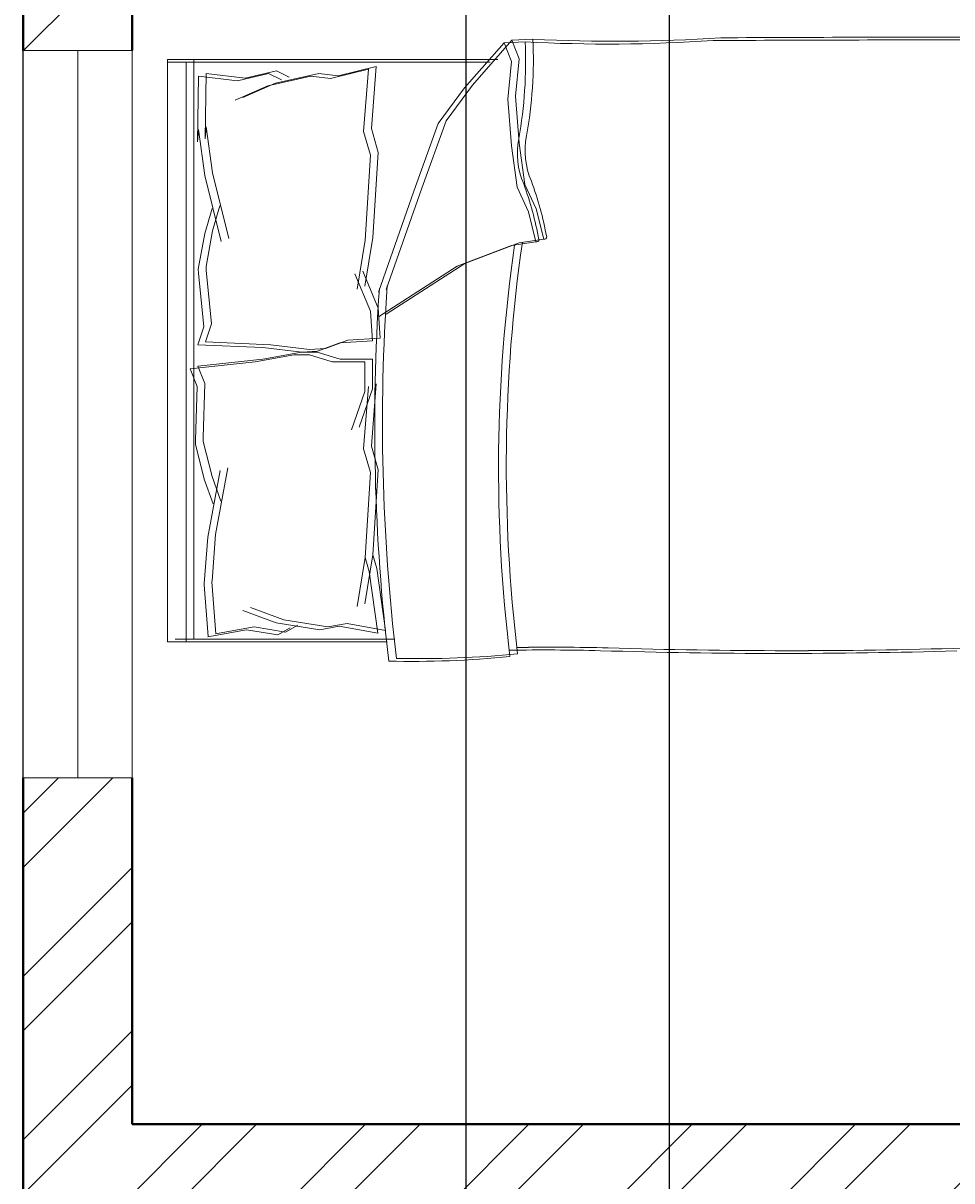
# Model space of a CAD drawing. Units: inches. Extents: x 1601 to 2297, y 1496 to 2631.
# Tile 33 of 57: x 1686 to 1763, y 2141 to 2236. Entities that reach past the tile are written whole.
import ezdxf

# ---------------------------------------------------------------- set-up
doc = ezdxf.new("R2010")
doc.units = ezdxf.units.IN
for name, color, linetype, lineweight in [('A-ANNO-DIMS', 2, 'Continuous', 18), ('A-FURN', 8, 'Continuous', 18), ('A-GLAZ', 161, 'Continuous', 20), ('A-WALL', 7, 'Continuous', 40), ('A-WALL-PATT', 215, 'Continuous', 13)]:
    doc.layers.add(name, color=color, linetype=linetype, lineweight=lineweight)
doc.styles.get("Standard").update_dxf_attribs({"font": 'arial.ttf'})
doc.dimstyles.get("Standard").update_dxf_attribs({"dimtxt": 0.18, "dimasz": 0.18, "dimexe": 0.18, "dimexo": 0.0625, "dimgap": 0.09, "dimtad": 0, "dimtih": 1, "dimtoh": 1, "dimdec": 4, "dimzin": 0, "dimdsep": 46, "dimtxsty": 'Standard', "dimcen": 0.09, "dimadec": 0, "dimazin": 0, "dimtfac": 1, "dimtdec": 4, "dimtofl": 0, "dimtmove": 0, "dimatfit": 3, "dimfxl": 1, "dimtolj": 1, "dimtzin": 0, "dimarcsym": 0})

# ---------------------------------------------------------------- blocks, each defined once
blk = doc.blocks.new('BED-DOUBLE')
for p, q in [((27.746, 52.867), (24.495, 49.162)), ((27.746, 52.867), (24.495, 49.162)), ((27.746, 52.867), (24.495, 49.162)), ((27.746, 52.867), (24.495, 49.162)), ((28.385, 53.096), (25.135, 49.39)), ((28.385, 53.096), (25.135, 49.39)), ((28.385, 53.096), (25.135, 49.39)), ((28.385, 53.096), (25.135, 49.39)), ((29.49, 52.947), (27.746, 52.867, 3.871)), ((29.49, 52.947), (27.746, 52.867, 3.871)), ((29.49, 52.947), (27.746, 52.867, 3.871)), ((29.49, 52.947), (27.746, 52.867, 3.871)), ((28.365, 51.33), (27.746, 52.867)), ((28.365, 51.33), (27.746, 52.867)), ((28.365, 51.33), (27.746, 52.867)), ((28.365, 51.33), (27.746, 52.867)), ((30.13, 53.175), (28.385, 53.096, 3.871)), ((30.13, 53.175), (28.385, 53.096, 3.871)), ((30.13, 53.175), (28.385, 53.096, 3.871)), ((30.13, 53.175), (28.385, 53.096, 3.871)), ((29.004, 51.559), (28.385, 53.096)), ((29.004, 51.558), (28.385, 53.096)), ((29.004, 51.559), (28.385, 53.096)), ((29.004, 51.558), (28.385, 53.096)), ((28.695, 48.461), (29.004, 51.559)), ((28.695, 48.461), (29.004, 51.559)), ((28.695, 48.461), (29.004, 51.558)), ((28.695, 48.461), (29.004, 51.558)), ((0, 51.494), (0.639, 51.493)), ((0, 3.475), (0, 51.494)), ((0, 51.494), (0.639, 51.493)), ((0, 3.475), (0, 51.494)), ((0, 51.265), (26.61, 51.265)), ((0, 51.265), (26.61, 51.265)), ((0, 51.265), (26.61, 51.265)), ((0, 51.265), (26.61, 51.265)), ((0.639, 51.494), (27.249, 51.494)), ((0.639, 51.494), (27.249, 51.494)), ((0.639, 51.493), (27.249, 51.493)), ((0.639, 51.493), (27.249, 51.493)), ((1.533, 3.475), (1.533, 51.265)), ((1.533, 3.475), (1.533, 51.265)), ((1.533, 3.475), (1.533, 51.265)), ((1.533, 3.475), (1.533, 51.265)), ((2.173, 3.703), (2.173, 51.494)), ((2.173, 3.703), (2.173, 51.494)), ((2.173, 3.703), (2.173, 51.493)), ((2.173, 3.703), (2.173, 51.493)), ((16.573, 50.698), (13.434, 49.923)), ((16.573, 50.698), (13.434, 49.922)), ((16.573, 50.698), (13.434, 49.923)), ((16.573, 50.698), (13.434, 49.922)), ((17.212, 50.926), (14.073, 50.151)), ((17.212, 50.926), (14.073, 50.151)), ((17.212, 50.926), (14.073, 50.151)), ((17.212, 50.926), (14.073, 50.151)), ((16.169, 45.566), (16.573, 50.698)), ((16.169, 45.566), (16.573, 50.698)), ((16.169, 45.566), (16.573, 50.698)), ((16.169, 45.566), (16.573, 50.698)), ((16.808, 45.795), (17.212, 50.926)), ((16.808, 45.794), (17.212, 50.926)), ((16.808, 45.795), (17.212, 50.926)), ((16.808, 45.794), (17.212, 50.926)), ((28.055, 48.233), (28.365, 51.33)), ((28.055, 48.233), (28.365, 51.33)), ((28.055, 48.233), (28.365, 51.33)), ((28.055, 48.233), (28.365, 51.33)), ((2.557, 50.112), (2.46, 44.709)), ((2.557, 50.112), (2.46, 44.709)), ((2.557, 50.111), (2.46, 44.709)), ((2.557, 50.111), (2.46, 44.709)), ((2.557, 50.112), (5.768, 49.733)), ((2.557, 50.112), (5.768, 49.733)), ((2.557, 50.111), (5.768, 49.733)), ((2.557, 50.111), (5.768, 49.733)), ((3.196, 50.34), (3.099, 44.938)), ((3.196, 50.34), (3.099, 44.938)), ((3.196, 50.34), (3.099, 44.938)), ((3.196, 50.34), (3.099, 44.938)), ((3.196, 50.34), (6.407, 49.961)), ((3.196, 50.34), (6.407, 49.961)), ((3.196, 50.34), (6.407, 49.961)), ((3.196, 50.34), (6.407, 49.961)), ((5.768, 49.733), (8.338, 50.328)), ((5.768, 49.733), (8.338, 50.328)), ((5.768, 49.733), (8.338, 50.328)), ((5.768, 49.733), (8.338, 50.328)), ((6.407, 49.961), (8.977, 50.557)), ((6.407, 49.961), (8.977, 50.557)), ((6.407, 49.961), (8.977, 50.556)), ((6.407, 49.961), (8.977, 50.556)), ((11.829, 50.112), (8.257, 49.309)), ((11.829, 50.112), (8.257, 49.309)), ((11.829, 50.112), (8.257, 49.309)), ((11.829, 50.112), (8.257, 49.309)), ((8.338, 50.328), (9.384, 49.814)), ((8.338, 50.328), (9.384, 49.814)), ((8.338, 50.328), (9.384, 49.814)), ((8.338, 50.328), (9.384, 49.814)), ((12.468, 50.34), (8.896, 49.538)), ((12.468, 50.34), (8.896, 49.537)), ((12.468, 50.34), (8.896, 49.538)), ((12.468, 50.34), (8.896, 49.537)), ((8.977, 50.557), (10.024, 50.043)), ((8.977, 50.557), (10.024, 50.043)), ((8.977, 50.556), (10.024, 50.042)), ((8.977, 50.556), (10.024, 50.042)), ((13.434, 49.923), (11.829, 50.112)), ((13.434, 49.922), (11.829, 50.112)), ((13.434, 49.923), (11.829, 50.112)), ((13.434, 49.922), (11.829, 50.112)), ((14.073, 50.151), (12.468, 50.34)), ((14.073, 50.151), (12.468, 50.34)), ((14.073, 50.151), (12.468, 50.34)), ((14.073, 50.151), (12.468, 50.34)), ((8.257, 49.309), (5.578, 48.128)), ((8.257, 49.309), (5.578, 48.128)), ((8.257, 49.309), (5.578, 48.128)), ((8.257, 49.309), (5.578, 48.128)), ((8.896, 49.538), (6.218, 48.356)), ((8.896, 49.538), (6.218, 48.356)), ((8.896, 49.537), (6.218, 48.356)), ((8.896, 49.537), (6.218, 48.356)), ((24.495, 49.162), (22.329, 46.219)), ((24.495, 49.162), (22.329, 46.219)), ((24.495, 49.162), (22.329, 46.219)), ((24.495, 49.162), (22.329, 46.219)), ((25.135, 49.39), (22.968, 46.448)), ((25.135, 49.39), (22.968, 46.448)), ((25.135, 49.39), (22.968, 46.448)), ((25.135, 49.39), (22.968, 46.448)), ((28.365, 44.361), (28.055, 48.233)), ((28.365, 44.361), (28.055, 48.233)), ((28.365, 44.361), (28.055, 48.233)), ((28.365, 44.361), (28.055, 48.233)), ((29.004, 44.589), (28.695, 48.461)), ((29.004, 44.589), (28.695, 48.461)), ((29.004, 44.589), (28.695, 48.461)), ((29.004, 44.589), (28.695, 48.461)), ((3.099, 44.938), (3.181, 45.941)), ((3.099, 44.938), (3.181, 45.941)), ((3.099, 44.938), (3.181, 45.94)), ((3.099, 44.938), (3.181, 45.94)), ((3.181, 45.941), (3.709, 42.143)), ((3.181, 45.941), (3.709, 42.143)), ((3.181, 45.94), (3.709, 42.142)), ((3.181, 45.94), (3.709, 42.142)), ((22.329, 46.219), (20.316, 40.644)), ((22.329, 46.219), (20.316, 40.644)), ((22.329, 46.219), (20.317, 40.644)), ((22.329, 46.219), (20.317, 40.644)), ((22.968, 46.448), (20.956, 40.872)), ((22.968, 46.448), (20.956, 40.872)), ((22.968, 46.448), (20.956, 40.872)), ((22.968, 46.448), (20.956, 40.872)), ((2.46, 44.709), (2.542, 45.712)), ((2.46, 44.709), (2.542, 45.712)), ((2.46, 44.709), (2.542, 45.712)), ((2.46, 44.709), (2.542, 45.712)), ((2.542, 45.712), (3.069, 41.914)), ((2.542, 45.712), (3.069, 41.914)), ((2.542, 45.712), (3.069, 41.914)), ((2.542, 45.712), (3.069, 41.914)), ((16.726, 43.606), (16.169, 45.566)), ((16.726, 43.606), (16.169, 45.566)), ((16.726, 43.606), (16.169, 45.566)), ((16.726, 43.606), (16.169, 45.566)), ((17.365, 43.834), (16.808, 45.795)), ((17.365, 43.834), (16.808, 45.795)), ((17.365, 43.834), (16.808, 45.794)), ((17.365, 43.834), (16.808, 45.794)), ((28.829, 40.954), (28.365, 44.361)), ((28.829, 40.953), (28.365, 44.361)), ((28.829, 40.954), (28.365, 44.361)), ((28.829, 40.953), (28.365, 44.361)), ((29.468, 41.182), (29.004, 44.589)), ((29.469, 41.182), (29.004, 44.589)), ((29.468, 41.182), (29.004, 44.589)), ((29.469, 41.182), (29.004, 44.589)), ((16.295, 36.596), (16.726, 43.606)), ((16.295, 36.596), (16.726, 43.606)), ((16.295, 36.596), (16.726, 43.606)), ((16.295, 36.596), (16.726, 43.606)), ((16.934, 36.824), (17.365, 43.834)), ((16.934, 36.824), (17.365, 43.834)), ((16.934, 36.824), (17.365, 43.834)), ((16.934, 36.824), (17.365, 43.834)), ((3.709, 42.143), (5.061, 36.723)), ((3.709, 42.143), (5.061, 36.723)), ((3.709, 42.142), (5.061, 36.723)), ((3.709, 42.142), (5.061, 36.723)), ((3.069, 41.914), (4.422, 36.495)), ((3.069, 41.914), (4.422, 36.495)), ((3.069, 41.914), (4.422, 36.495)), ((3.069, 41.914), (4.422, 36.495)), ((30.397, 39.169), (29.468, 41.182)), ((30.397, 39.169), (29.468, 41.182)), ((30.397, 39.168), (29.469, 41.182)), ((30.397, 39.168), (29.469, 41.182)), ((20.316, 40.644), (17.383, 32.306)), ((20.317, 40.644), (17.383, 32.306)), ((20.316, 40.644), (17.383, 32.306)), ((20.317, 40.644), (17.383, 32.306)), ((20.956, 40.872), (18.022, 32.534)), ((20.956, 40.872), (18.022, 32.534)), ((20.956, 40.872), (18.022, 32.534)), ((20.956, 40.872), (18.022, 32.534)), ((29.758, 38.94), (28.829, 40.954)), ((29.758, 38.94), (28.829, 40.954)), ((29.758, 38.94), (28.829, 40.953)), ((29.758, 38.94), (28.829, 40.953)), ((3.673, 39.2), (3.078, 37.135)), ((3.673, 39.2), (3.078, 37.135)), ((3.673, 39.2), (3.078, 37.135)), ((3.673, 39.2), (3.078, 37.135)), ((4.313, 39.428), (3.717, 37.363)), ((4.313, 39.428), (3.717, 37.363)), ((4.313, 39.428), (3.718, 37.363)), ((4.313, 39.428), (3.718, 37.363)), ((31.016, 36.691), (30.397, 39.169)), ((31.016, 36.691), (30.397, 39.169)), ((31.016, 36.691), (30.397, 39.168)), ((31.016, 36.691), (30.397, 39.168)), ((30.377, 36.462), (29.758, 38.94)), ((30.377, 36.462), (29.758, 38.94)), ((30.377, 36.462), (29.758, 38.94)), ((30.377, 36.462), (29.758, 38.94)), ((3.717, 37.363), (3.176, 34.433)), ((3.718, 37.363), (3.176, 34.433)), ((3.717, 37.363), (3.176, 34.433)), ((3.718, 37.363), (3.176, 34.433)), ((3.078, 37.135), (2.537, 34.204)), ((3.078, 37.135), (2.537, 34.204)), ((3.078, 37.135), (2.537, 34.204)), ((3.078, 37.135), (2.537, 34.204)), ((15.628, 32.564), (16.295, 36.596)), ((15.628, 32.564), (16.295, 36.596)), ((15.628, 32.564), (16.295, 36.596)), ((15.628, 32.564), (16.295, 36.596)), ((16.268, 32.792), (16.934, 36.824)), ((16.268, 32.792), (16.934, 36.824)), ((16.268, 32.792), (16.934, 36.824)), ((16.268, 32.792), (16.934, 36.824)), ((24.516, 34.677), (29.004, 36.381)), ((24.516, 34.677), (29.004, 36.381)), ((24.516, 34.677), (29.004, 36.381)), ((24.516, 34.677), (29.004, 36.381)), ((28.365, 36.153), (30.377, 36.462)), ((28.365, 36.152), (30.377, 36.462)), ((28.365, 36.153), (30.377, 36.462)), ((28.365, 36.152), (30.377, 36.462)), ((29.004, 36.381), (31.016, 36.691)), ((29.004, 36.381), (31.016, 36.691)), ((29.004, 36.381), (31.016, 36.691)), ((29.004, 36.381), (31.016, 36.691)), ((23.876, 34.449), (28.365, 36.153)), ((23.876, 34.449), (28.365, 36.153)), ((23.876, 34.449), (28.365, 36.152)), ((23.876, 34.449), (28.365, 36.152)), ((3.176, 34.433), (3.196, 34.112)), ((3.176, 34.433), (3.196, 34.112)), ((3.176, 34.433), (3.196, 34.112)), ((3.176, 34.433), (3.196, 34.112)), ((17.383, 30.259), (23.876, 34.449)), ((17.383, 30.259), (23.876, 34.449)), ((17.383, 30.259), (23.876, 34.449)), ((17.383, 30.259), (23.876, 34.449)), ((18.022, 30.487), (24.516, 34.677)), ((18.022, 30.487), (24.516, 34.677)), ((18.022, 30.487), (24.516, 34.677)), ((18.022, 30.487), (24.516, 34.677)), ((2.537, 34.204), (2.557, 33.883)), ((2.537, 34.204), (2.557, 33.883)), ((2.537, 34.204), (2.557, 33.883)), ((2.537, 34.204), (2.557, 33.883)), ((2.557, 33.883), (2.979, 29.456)), ((2.557, 33.883), (2.979, 29.455)), ((2.557, 33.883), (2.979, 29.456)), ((2.557, 33.883), (2.979, 29.455)), ((3.196, 34.112), (3.618, 29.684)), ((3.196, 34.112), (3.618, 29.684)), ((3.196, 34.112), (3.618, 29.684)), ((3.196, 34.112), (3.618, 29.684)), ((16.739, 30.75), (15.454, 33.821)), ((16.739, 30.75), (15.454, 33.821)), ((16.739, 30.75), (15.454, 33.82)), ((16.739, 30.75), (15.454, 33.82)), ((17.379, 30.978), (16.094, 34.049)), ((17.379, 30.978), (16.094, 34.049)), ((17.379, 30.978), (16.094, 34.049)), ((17.379, 30.978), (16.094, 34.049)), ((16.893, 28.297), (16.739, 30.75)), ((16.893, 28.297), (16.739, 30.75)), ((16.893, 28.297), (16.739, 30.75)), ((16.893, 28.297), (16.739, 30.75)), ((17.532, 28.526), (17.379, 30.978)), ((17.532, 28.525), (17.379, 30.978)), ((17.532, 28.526), (17.379, 30.978)), ((17.532, 28.525), (17.379, 30.978)), ((3.618, 29.684), (3.131, 28.205)), ((3.618, 29.684), (3.131, 28.205)), ((3.618, 29.684), (3.131, 28.205)), ((3.618, 29.684), (3.131, 28.205)), ((2.979, 29.456), (2.492, 27.977)), ((2.979, 29.456), (2.492, 27.977)), ((2.979, 29.455), (2.492, 27.976)), ((2.979, 29.455), (2.492, 27.976)), ((2.492, 27.977), (7.867, 27.733)), ((2.492, 27.977), (7.867, 27.733)), ((2.492, 27.976), (7.867, 27.733)), ((2.492, 27.976), (7.867, 27.733)), ((3.131, 28.205), (8.506, 27.962)), ((3.131, 28.205), (8.506, 27.961)), ((3.131, 28.205), (8.506, 27.962)), ((3.131, 28.205), (8.506, 27.961)), ((7.867, 27.733), (11.078, 27.355)), ((7.867, 27.733), (11.078, 27.354)), ((7.867, 27.733), (11.078, 27.355)), ((7.867, 27.733), (11.078, 27.354)), ((8.506, 27.962), (11.717, 27.583)), ((8.506, 27.962), (11.717, 27.583)), ((8.506, 27.961), (11.717, 27.583)), ((8.506, 27.961), (11.717, 27.583)), ((12.377, 27.436), (14.216, 28.13)), ((12.377, 27.436), (14.217, 28.13)), ((12.377, 27.436), (14.216, 28.13)), ((12.377, 27.436), (14.217, 28.13)), ((13.016, 27.664), (14.856, 28.359)), ((13.016, 27.664), (14.856, 28.359)), ((13.016, 27.664), (14.856, 28.358)), ((13.016, 27.664), (14.856, 28.358)), ((14.216, 28.13), (16.893, 28.297)), ((14.216, 28.13), (16.893, 28.297)), ((14.217, 28.13), (16.893, 28.297)), ((14.217, 28.13), (16.893, 28.297)), ((14.856, 28.359), (17.532, 28.526)), ((14.856, 28.359), (17.532, 28.526)), ((14.856, 28.358), (17.532, 28.525)), ((14.856, 28.358), (17.532, 28.525)), ((2.509, 26.211), (7.859, 26.789)), ((2.509, 26.21), (7.859, 26.789)), ((2.509, 26.211), (7.859, 26.789)), ((2.509, 26.21), (7.859, 26.789)), ((7.22, 26.561), (10.401, 27.139)), ((7.22, 26.56), (10.401, 27.139)), ((7.22, 26.561), (10.401, 27.139)), ((7.22, 26.56), (10.401, 27.139)), ((7.859, 26.789), (11.04, 27.367)), ((7.859, 26.789), (11.04, 27.367)), ((7.859, 26.789), (11.04, 27.367)), ((7.859, 26.789), (11.04, 27.367)), ((10.401, 27.139), (11.702, 27.139)), ((10.401, 27.139), (11.702, 27.139)), ((10.401, 27.139), (11.702, 27.139)), ((10.401, 27.139), (11.702, 27.139)), ((11.04, 27.367), (12.341, 27.367)), ((11.04, 27.367), (12.341, 27.367)), ((11.04, 27.367), (12.341, 27.367)), ((11.04, 27.367), (12.341, 27.367)), ((11.078, 27.355), (12.377, 27.436)), ((11.078, 27.354), (12.377, 27.436)), ((11.078, 27.355), (12.377, 27.436)), ((11.078, 27.354), (12.377, 27.436)), ((11.702, 27.139), (13.582, 26.561)), ((11.702, 27.139), (13.582, 26.56)), ((11.702, 27.139), (13.582, 26.561)), ((11.702, 27.139), (13.582, 26.56)), ((11.717, 27.583), (13.016, 27.664)), ((11.717, 27.583), (13.016, 27.664)), ((11.717, 27.583), (13.016, 27.664)), ((11.717, 27.583), (13.016, 27.664)), ((12.341, 27.367), (14.221, 26.789)), ((12.341, 27.367), (14.221, 26.789)), ((12.341, 27.367), (14.221, 26.789)), ((12.341, 27.367), (14.221, 26.789)), ((14.221, 26.789), (16.902, 26.789)), ((14.221, 26.789), (16.902, 26.789)), ((14.221, 26.789), (16.902, 26.789)), ((14.221, 26.789), (16.902, 26.789)), ((16.902, 26.789), (16.902, 24.332)), ((16.902, 26.789), (16.902, 24.331)), ((16.902, 26.789), (16.902, 24.332)), ((16.902, 26.789), (16.902, 24.331)), ((1.87, 25.982), (7.22, 26.561)), ((1.87, 25.982), (7.22, 26.561)), ((1.87, 25.982), (7.22, 26.56)), ((1.87, 25.982), (7.22, 26.56)), ((2.448, 24.537), (1.87, 25.982)), ((2.448, 24.537), (1.87, 25.982)), ((2.448, 24.537), (1.87, 25.982)), ((2.448, 24.537), (1.87, 25.982)), ((3.088, 24.765), (2.509, 26.211)), ((3.088, 24.765), (2.509, 26.211)), ((3.088, 24.765), (2.509, 26.21)), ((3.088, 24.765), (2.509, 26.21)), ((13.582, 26.561), (16.263, 26.561)), ((13.582, 26.561), (16.263, 26.561)), ((13.582, 26.56), (16.263, 26.56)), ((13.582, 26.56), (16.263, 26.56)), ((16.263, 26.561), (16.263, 24.103)), ((16.263, 26.561), (16.263, 24.103)), ((16.263, 26.56), (16.263, 24.103)), ((16.263, 26.56), (16.263, 24.103)), ((2.304, 20.091), (2.448, 24.537)), ((2.304, 20.091), (2.448, 24.537)), ((2.304, 20.091), (2.448, 24.537)), ((2.304, 20.091), (2.448, 24.537)), ((2.943, 20.32), (3.088, 24.765)), ((2.943, 20.319), (3.088, 24.765)), ((2.943, 20.32), (3.088, 24.765)), ((2.943, 20.319), (3.088, 24.765)), ((16.263, 24.103), (15.172, 20.959)), ((16.263, 24.103), (15.172, 20.958)), ((16.263, 24.103), (15.172, 20.959)), ((16.263, 24.103), (15.172, 20.958)), ((16.902, 24.332), (15.811, 21.187)), ((16.902, 24.332), (15.811, 21.187)), ((16.902, 24.331), (15.811, 21.187)), ((16.902, 24.331), (15.811, 21.187)), ((16.169, 19.384), (16.573, 24.516)), ((16.169, 19.384), (16.573, 24.516)), ((16.169, 19.383), (16.573, 24.515)), ((16.169, 19.383), (16.573, 24.515)), ((16.808, 19.612), (17.212, 24.744)), ((16.808, 19.612), (17.212, 24.744)), ((16.808, 19.612), (17.212, 24.744)), ((16.808, 19.612), (17.212, 24.744)), ((2.304, 19.77), (2.304, 20.091)), ((2.304, 19.769), (2.304, 20.091)), ((2.304, 19.77), (2.304, 20.091)), ((2.304, 19.769), (2.304, 20.091)), ((2.943, 19.998), (2.943, 20.32)), ((2.943, 19.998), (2.943, 20.32)), ((2.943, 19.998), (2.943, 20.319)), ((2.943, 19.998), (2.943, 20.319)), ((3.027, 16.878), (2.304, 19.77)), ((3.027, 16.878), (2.304, 19.77)), ((3.027, 16.878), (2.304, 19.769)), ((3.027, 16.878), (2.304, 19.769)), ((3.666, 17.107), (2.943, 19.998)), ((3.666, 17.107), (2.943, 19.998)), ((3.666, 17.107), (2.943, 19.998)), ((3.666, 17.107), (2.943, 19.998)), ((16.726, 17.423), (16.169, 19.384)), ((16.726, 17.423), (16.169, 19.384)), ((16.726, 17.423), (16.169, 19.383)), ((16.726, 17.423), (16.169, 19.383)), ((17.365, 17.652), (16.808, 19.612)), ((17.365, 17.651), (16.808, 19.612)), ((17.365, 17.652), (16.808, 19.612)), ((17.365, 17.651), (16.808, 19.612)), ((3.316, 12.108), (4.328, 17.601)), ((3.316, 12.108), (4.328, 17.601)), ((3.316, 12.108), (4.328, 17.601)), ((3.316, 12.108), (4.328, 17.601)), ((3.955, 12.336), (4.967, 17.83)), ((3.955, 12.336), (4.967, 17.83)), ((3.955, 12.336), (4.967, 17.829)), ((3.955, 12.336), (4.967, 17.829)), ((16.295, 10.413), (16.726, 17.423)), ((16.295, 10.413), (16.726, 17.423)), ((16.295, 10.413), (16.726, 17.423)), ((16.295, 10.413), (16.726, 17.423)), ((16.934, 10.642), (17.365, 17.652)), ((16.934, 10.642), (17.365, 17.652)), ((16.934, 10.642), (17.365, 17.651)), ((16.934, 10.642), (17.365, 17.651)), ((3.75, 14.855), (3.027, 16.878)), ((3.75, 14.854), (3.027, 16.878)), ((3.75, 14.855), (3.027, 16.878)), ((3.75, 14.854), (3.027, 16.878)), ((4.389, 15.083), (3.666, 17.107)), ((4.389, 15.083), (3.666, 17.107)), ((4.389, 15.083), (3.666, 17.107)), ((4.389, 15.083), (3.666, 17.107)), ((3.027, 8.285), (3.316, 12.108)), ((3.027, 8.284), (3.316, 12.108)), ((3.027, 8.285), (3.316, 12.108)), ((3.027, 8.284), (3.316, 12.108)), ((3.666, 8.513), (3.955, 12.336)), ((3.666, 8.513), (3.955, 12.336)), ((3.666, 8.513), (3.955, 12.336)), ((3.666, 8.513), (3.955, 12.336)), ((16.268, 6.61), (16.934, 10.642)), ((16.268, 6.61), (16.934, 10.642)), ((16.268, 6.61), (16.934, 10.642)), ((16.268, 6.61), (16.934, 10.642)), ((16.934, 10.642), (17.257, 9.509)), ((16.934, 10.642), (17.257, 9.508)), ((16.934, 10.642), (17.257, 9.509)), ((16.934, 10.642), (17.257, 9.508)), ((15.628, 6.382), (16.295, 10.413)), ((15.628, 6.381), (16.295, 10.413)), ((15.628, 6.382), (16.295, 10.413)), ((15.628, 6.381), (16.295, 10.413)), ((16.295, 10.413), (16.618, 9.28)), ((16.295, 10.413), (16.618, 9.28)), ((16.295, 10.413), (16.618, 9.28)), ((16.295, 10.413), (16.618, 9.28)), ((16.618, 9.28), (17.341, 4.184)), ((16.618, 9.28), (17.341, 4.183)), ((16.618, 9.28), (17.341, 4.184)), ((16.618, 9.28), (17.341, 4.183)), ((17.257, 9.509), (17.98, 4.412)), ((17.257, 9.509), (17.98, 4.412)), ((17.257, 9.508), (17.98, 4.412)), ((17.257, 9.508), (17.98, 4.412)), ((3.009, 8.179), (3.027, 8.285)), ((3.009, 8.179), (3.027, 8.285)), ((3.009, 8.179), (3.027, 8.284)), ((3.009, 8.179), (3.027, 8.284)), ((3.338, 3.898), (3.009, 8.179)), ((3.338, 3.898), (3.009, 8.179)), ((3.338, 3.898), (3.009, 8.179)), ((3.338, 3.898), (3.009, 8.179)), ((3.648, 8.408), (3.666, 8.513)), ((3.648, 8.407), (3.666, 8.513)), ((3.648, 8.408), (3.666, 8.513)), ((3.648, 8.407), (3.666, 8.513)), ((3.977, 4.127), (3.648, 8.408)), ((3.977, 4.127), (3.648, 8.408)), ((3.977, 4.127), (3.648, 8.407)), ((3.977, 4.127), (3.648, 8.407)), ((8.955, 5.051), (6.208, 6.063)), ((8.955, 5.051), (6.208, 6.063)), ((8.955, 5.051), (6.208, 6.063)), ((8.955, 5.051), (6.208, 6.063)), ((9.594, 5.279), (6.847, 6.291)), ((9.594, 5.279), (6.847, 6.291)), ((9.594, 5.279), (6.847, 6.291)), ((9.594, 5.279), (6.847, 6.291)), ((12.57, 4.473), (8.955, 5.051)), ((12.57, 4.472), (8.955, 5.051)), ((12.57, 4.473), (8.955, 5.051)), ((12.57, 4.472), (8.955, 5.051)), ((13.209, 4.701), (9.594, 5.279)), ((13.209, 4.701), (9.594, 5.279)), ((13.209, 4.701), (9.594, 5.279)), ((13.209, 4.701), (9.594, 5.279)), ((9.739, 4.267), (10.751, 4.846)), ((9.739, 4.267), (10.751, 4.846)), ((9.739, 4.267), (10.751, 4.845)), ((9.739, 4.267), (10.751, 4.845)), ((14.799, 4.99), (13.209, 4.701)), ((14.799, 4.99), (13.209, 4.701)), ((14.799, 4.99), (13.209, 4.701)), ((14.799, 4.99), (13.209, 4.701)), ((17.98, 4.412), (14.799, 4.99)), ((17.98, 4.412), (14.799, 4.99)), ((17.98, 4.412), (14.799, 4.99)), ((17.98, 4.412), (14.799, 4.99)), ((3.316, 3.894), (6.497, 4.473)), ((3.316, 3.894), (6.497, 4.473)), ((3.316, 3.894), (6.497, 4.472)), ((3.316, 3.894), (6.497, 4.472)), ((3.955, 4.123), (7.136, 4.701)), ((3.955, 4.123), (7.136, 4.701)), ((3.955, 4.123), (7.136, 4.701)), ((3.955, 4.123), (7.136, 4.701)), ((6.497, 4.473), (9.099, 4.039)), ((6.497, 4.473), (9.099, 4.039)), ((6.497, 4.472), (9.099, 4.039)), ((6.497, 4.472), (9.099, 4.039)), ((7.136, 4.701), (9.739, 4.267)), ((7.136, 4.701), (9.739, 4.267)), ((7.136, 4.701), (9.739, 4.267)), ((7.136, 4.701), (9.739, 4.267)), ((9.099, 4.039), (10.112, 4.617)), ((9.099, 4.039), (10.112, 4.617)), ((9.099, 4.039), (10.112, 4.617)), ((9.099, 4.039), (10.112, 4.617)), ((14.16, 4.762), (12.57, 4.473)), ((14.16, 4.762), (12.57, 4.472)), ((14.16, 4.762), (12.57, 4.473)), ((14.16, 4.762), (12.57, 4.472)), ((17.341, 4.184), (14.16, 4.762)), ((17.341, 4.183), (14.16, 4.762)), ((17.341, 4.184), (14.16, 4.762)), ((17.341, 4.183), (14.16, 4.762)), ((18.11, 3.475), (0, 3.475)), ((18.11, 3.475), (0, 3.475)), ((18.11, 3.475), (0, 3.475)), ((18.11, 3.475), (0, 3.475)), ((18.75, 3.703), (0.639, 3.703)), ((18.75, 3.703), (0.639, 3.703)), ((18.75, 3.703), (0.639, 3.703)), ((18.75, 3.703), (0.639, 3.703))]:
    blk.add_line(p, q)
for centre, radius, start, end in [((-6.656, 51.327), 36.183, 349.87628, 2.56571), ((-6.656, 51.327), 36.183, 349.87628, 2.56571), ((-6.656, 51.327), 36.183, 349.87628, 2.56571), ((-6.656, 51.327), 36.183, 349.87628, 2.56571), ((36.315, 182.266), 129.499, 266.97912, 273.83645), ((36.315, 182.265), 129.499, 266.97912, 273.83645), ((36.315, 182.266), 129.499, 266.97912, 273.83645), ((36.315, 182.265), 129.499, 266.97912, 273.83645), ((-6.017, 51.555), 36.183, 349.87628, 2.56571), ((-6.017, 51.555), 36.183, 349.87628, 2.56571), ((-6.017, 51.555), 36.183, 349.87628, 2.56571), ((-6.017, 51.555), 36.183, 349.87628, 2.56571), ((36.954, 182.494), 129.499, 266.97912, 273.83645), ((36.954, 182.494), 129.499, 266.97912, 273.83645), ((36.954, 182.494), 129.499, 266.97912, 273.83645), ((36.954, 182.494), 129.499, 266.97912, 273.83645), ((67.821, -4508.744), 4561.858, 90.002168, 90.286887), ((67.821, -4508.744), 4561.858, 90.002168, 90.286887), ((67.821, -4508.744), 4561.858, 90.002168, 90.286887), ((67.821, -4508.744), 4561.858, 90.002168, 90.286887), ((68.461, -4508.515), 4561.858, 90.002168, 90.286887), ((68.461, -4508.515), 4561.858, 90.002168, 90.286887), ((68.461, -4508.516), 4561.858, 90.002168, 90.286887), ((68.461, -4508.516), 4561.858, 90.002168, 90.286887), ((35.066, 43.743), 6.224, 168.6608, 203.73842), ((35.066, 43.743), 6.224, 168.6608, 203.73842), ((35.066, 43.743), 6.224, 168.6608, 203.73842), ((35.066, 43.743), 6.224, 168.6608, 203.73842), ((35.705, 43.972), 6.224, 168.6608, 203.73842), ((35.705, 43.971), 6.224, 168.6608, 203.73842), ((35.705, 43.972), 6.224, 168.6608, 203.73842), ((35.705, 43.971), 6.224, 168.6608, 203.73842), ((1.482, 31.154), 29.654, 10.66171, 19.88058), ((1.482, 31.154), 29.654, 10.66171, 19.88058), ((1.482, 31.153), 29.654, 10.66171, 19.88058), ((1.482, 31.153), 29.654, 10.66171, 19.88058), ((2.121, 31.382), 29.654, 10.66171, 19.88058), ((2.121, 31.382), 29.654, 10.66171, 19.88058), ((2.121, 31.382), 29.654, 10.66171, 19.88058), ((2.121, 31.382), 29.654, 10.66171, 19.88058), ((156.955, 17.984), 129.02, 171.78449, 186.90062), ((156.955, 17.984), 129.02, 171.78449, 186.90062), ((156.955, 17.984), 129.02, 171.78449, 186.90062), ((156.955, 17.984), 129.02, 171.78449, 186.90062), ((30.439, 36.636), 0.185, 250.24637, 1.13765), ((30.439, 36.636), 0.185, 250.24637, 1.13765), ((30.439, 36.636), 0.185, 250.24637, 1.13765), ((30.439, 36.636), 0.185, 250.24637, 1.13765), ((31.079, 36.864), 0.185, 250.24637, 1.13765), ((31.079, 36.864), 0.185, 250.24637, 1.13765), ((31.079, 36.864), 0.185, 250.24637, 1.13765), ((31.079, 36.864), 0.185, 250.24637, 1.13765), ((156.316, 17.756), 129.02, 171.78449, 186.90062), ((156.316, 17.755), 129.02, 171.78449, 186.90062), ((156.316, 17.756), 129.02, 171.78449, 186.90062), ((156.316, 17.755), 129.02, 171.78449, 186.90062), ((182.052, 21.359), 164.969, 176.08655, 186.78213), ((182.052, 21.359), 164.969, 176.08655, 186.78213), ((182.052, 21.358), 164.969, 176.08655, 186.78213), ((182.052, 21.358), 164.969, 176.08655, 186.78213), ((182.692, 21.587), 164.969, 176.08655, 186.78213), ((182.692, 21.587), 164.969, 176.08655, 186.78213), ((182.692, 21.587), 164.969, 176.08655, 186.78213), ((182.692, 21.587), 164.969, 176.08655, 186.78213), ((31.813, -167.079), 170.11, 88.4762, 91.00819), ((31.813, -167.08), 170.11, 88.4762, 91.00819), ((31.813, -167.079), 170.11, 88.4762, 91.00819), ((31.813, -167.08), 170.11, 88.4762, 91.00819), ((51.253, 485.051), 482.31, 268.22771, 271.71854), ((51.253, 485.05), 482.31, 268.22771, 271.71854), ((51.253, 485.051), 482.31, 268.22771, 271.71854), ((51.253, 485.05), 482.31, 268.22771, 271.71854), ((20.096, 85.162), 83.306, 268.72178, 275.60397), ((20.096, 85.161), 83.306, 268.72178, 275.60397), ((20.096, 85.162), 83.306, 268.72178, 275.60397), ((20.096, 85.161), 83.306, 268.72178, 275.60397), ((20.735, 85.39), 83.306, 268.72178, 275.60397), ((20.735, 85.39), 83.306, 268.72178, 275.60397), ((20.736, 85.39), 83.306, 268.72178, 275.60397), ((20.736, 85.39), 83.306, 268.72178, 275.60397), ((31.174, -167.308), 170.11, 88.4762, 91.00819), ((31.174, -167.308), 170.11, 88.4762, 91.00819), ((31.174, -167.308), 170.11, 88.4762, 91.00819), ((31.174, -167.308), 170.11, 88.4762, 91.00819), ((50.614, 484.822), 482.31, 268.22771, 271.71854), ((50.614, 484.822), 482.31, 268.22771, 271.71854), ((50.614, 484.822), 482.31, 268.22771, 271.71854), ((50.614, 484.822), 482.31, 268.22771, 271.71854)]:
    blk.add_arc(centre, radius, start, end)
blk = doc.blocks.new('WIN-60IN-JAMB9')
for p, q in [((4.5, 60), (0, 60)), ((0, 60), (9, 60)), ((0, 60), (0, 0)), ((4.5, 0), (4.5, 60)), ((9, 60), (9, 0)), ((0, 0), (9, 0)), ((9, 0), (4.5, 0))]:
    blk.add_line(p, q)
blk = doc.blocks.new('*D32')
at = {"layer": 'A-ANNO-DIMS', "color": 0, "lineweight": -2, "transparency": 16777216}
for p, q in [((1686.037, 2031.388), (1686.037, 2581.055)), ((1686.217, 2580.875), (1703.909, 2580.875)), ((1722.389, 2580.875), (1704.697, 2580.875)), ((1722.569, 2031.388), (1722.569, 2581.055))]:
    blk.add_line(p, q, dxfattribs=at)
at = {"layer": 'A-ANNO-DIMS', "color": 0, "transparency": 16777216}
for points in [[(1686.217, 2580.905), (1686.217, 2580.845), (1686.037, 2580.875)], [(1722.389, 2580.905), (1722.389, 2580.845), (1722.569, 2580.875)]]:
    blk.add_solid(points, dxfattribs=at)
at = {"layer": 'Defpoints', "color": 0, "transparency": 16777216}
for p in [(1722.569, 2580.875), (1686.037, 2031.325), (1722.569, 2031.325)]:
    blk.add_point(p, dxfattribs=at)
at = {"layer": 'A-ANNO-DIMS', "color": 0, "transparency": 16777216, "insert": (1704.303, 2580.875), "char_height": 0.18, "attachment_point": 5}
blk.add_mtext('\\A1;36.53', dxfattribs=at)
blk = doc.blocks.new('*D36')
at = {"layer": 'A-ANNO-DIMS', "color": 0, "lineweight": -2, "transparency": 16777216}
for p, q in [((1686.037, 1635.388), (1686.037, 2581.055)), ((1686.217, 2580.875), (1712.362, 2580.875)), ((1739.154, 2580.875), (1713.009, 2580.875)), ((1739.334, 1635.388), (1739.334, 2581.055))]:
    blk.add_line(p, q, dxfattribs=at)
at = {"layer": 'A-ANNO-DIMS', "color": 0, "transparency": 16777216}
for points in [[(1686.217, 2580.905), (1686.217, 2580.845), (1686.037, 2580.875)], [(1739.154, 2580.905), (1739.154, 2580.845), (1739.334, 2580.875)]]:
    blk.add_solid(points, dxfattribs=at)
at = {"layer": 'Defpoints', "color": 0, "transparency": 16777216}
for p in [(1739.334, 2580.875), (1686.037, 1635.325), (1739.334, 1635.325)]:
    blk.add_point(p, dxfattribs=at)
at = {"layer": 'A-ANNO-DIMS', "color": 0, "transparency": 16777216, "insert": (1712.685, 2580.875), "char_height": 0.18, "attachment_point": 5}
blk.add_mtext('\\A1;53.3', dxfattribs=at)

msp = doc.modelspace()

# ---------------------------------------------------------------- hatches: boundary and pattern name
at = {"layer": 'A-WALL-PATT'}
h = msp.add_hatch(dxfattribs=at)
h.set_pattern_fill('ANSI32', color=256)
h.paths.add_polyline_path([(1973.9371, 2211.3254), (1893.0373, 2211.3254), (1893.0373, 2287.8254), (1884.6167, 2287.8254), (1884.6167, 2285.5754), (1884.6167, 2283.3254), (1888.5373, 2283.3254), (1888.5373, 2145.3254), (1695.0373, 2145.3254), (1695.0373, 2173.8724), (1690.5373, 2173.8724), (1686.0373, 2173.8724), (1686.0373, 2136.3254), (1722.5687, 2136.3254), (1722.5687, 2117.4352), (1731.5687, 2117.4352), (1731.5687, 2136.3254), (1893.0373, 2136.3254), (1893.0373, 2202.3254), (1959.0373, 2202.3254), (1959.0373, 2182.1303), (1968.0373, 2182.1303), (1968.0373, 2202.3254), (1973.9371, 2202.3254)])
h.paths.add_polyline_path([(2094.0373, 2274.6364), (2096.4294, 2274.6364), (2096.4294, 2276.8864), (2096.4294, 2279.1364), (2094.0373, 2279.1364), (2094.0373, 2290.8254), (2094.0373, 2295.3254), (2089.5373, 2295.3254), (2089.5373, 2230.8254), (2035.5373, 2230.8254), (2035.5373, 2299.8254), (2031.0373, 2299.8254), (2031.0373, 2211.3254), (2023.0065, 2211.3254), (2023.0065, 2202.3254), (2031.0373, 2202.3254), (2031.0373, 2140.8254), (1968.0373, 2140.8254), (1968.0373, 2145.9106), (1963.5373, 2145.9106), (1959.0373, 2145.9106), (1959.0373, 2116.839), (1963.5373, 2116.839), (1968.0373, 2116.839), (1968.0373, 2131.8254), (2031.0373, 2131.8254), (2031.0373, 2094.3254), (2031.0373, 2085.3254), (2031.0373, 2056.8254), (1968.0373, 2056.8254), (1968.0373, 2070.4947), (1963.5373, 2070.4947), (1959.0373, 2070.4947), (1959.0373, 2040.3029), (1968.0373, 2040.3029), (1968.0373, 2047.8254), (2031.0373, 2047.8254), (2031.0373, 1983.3254), (2031.0373, 1978.8254), (2021.1979, 1978.8254), (2021.1979, 1974.3254), (2031.0373, 1974.3254), (2031.0373, 1954.3528), (2035.5373, 1954.3528), (2035.5373, 1974.3254), (2035.5373, 1981.8254), (2055.5513, 1981.8254), (2055.5513, 1986.3254), (2035.5373, 1986.3254), (2035.5373, 2047.8254), (2040.0373, 2047.8254), (2040.0373, 2085.3254), (2040.0373, 2094.3254), (2040.0373, 2140.8254), (2035.5373, 2140.8254), (2035.5373, 2226.3254), (2089.5373, 2226.3254), (2094.0373, 2226.3254)])
h.paths.add_polyline_path([(2226.0373, 2230.8254), (2134.5373, 2230.8254), (2134.5373, 2233.5437), (2130.0373, 2233.5437), (2130.0373, 2226.3254), (2134.5373, 2226.3254), (2226.0373, 2226.3254)])
h.paths.add_polyline_path([(1807.1169, 1573.5395), (2055.0405, 1573.5395), (2055.0405, 1610.6322), (1807.1169, 1610.6322)], flags=9)
h.paths.add_polyline_path([(1841.1631, 1712.7967), (1870.3957, 1712.7967), (1870.3957, 1731.454), (1841.1631, 1731.454)], flags=9)
h.paths.add_polyline_path([(2144.3862, 1772.185), (2191.0233, 1772.185), (2191.0233, 1790.8423), (2144.3862, 1790.8423)], flags=9)
h.paths.add_polyline_path([(2143.0128, 1827.3312), (2177.9958, 1827.3312), (2177.9958, 1845.9886), (2143.0128, 1845.9886)], flags=9)
h.paths.add_polyline_path([(2041.2439, 1833.5691), (2070.8516, 1833.5691), (2070.8516, 1852.2264), (2041.2439, 1852.2264)], flags=9)
h.paths.add_polyline_path([(2097.2791, 1947.0598), (2134.2061, 1947.0598), (2134.2061, 1965.7171), (2097.2791, 1965.7171)], flags=9)
h.paths.add_polyline_path([(2214.995, 1904.3124), (2214.995, 1942.2899), (2196.3376, 1942.2899), (2196.3376, 1904.3124)], flags=9)
h.paths.add_polyline_path([(2186.6284, 2043.8031), (2219.7935, 2043.8031), (2219.7935, 2062.4605), (2186.6284, 2062.4605)], flags=9)
h.paths.add_polyline_path([(2064.0877, 2031.616), (2097.4949, 2031.616), (2097.4949, 2050.2734), (2064.0877, 2050.2734)], flags=9)
h.paths.add_polyline_path([(1973.1349, 1986.0688), (2008.4009, 1986.0688), (2008.4009, 2004.7261), (1973.1349, 2004.7261)], flags=25)
h.paths.add_polyline_path([(1976.3676, 2106.9635), (2005.7469, 2106.9635), (2005.7469, 2125.6209), (1976.3676, 2125.6209)], flags=25)
h.paths.add_polyline_path([(1991.7852, 2180.4863), (2027.0513, 2180.4863), (2027.0513, 2199.1437), (1991.7852, 2199.1437)], flags=25)
h.paths.add_polyline_path([(2106.1801, 2187.9359), (2152.2101, 2187.9359), (2152.2101, 2206.5932), (2106.1801, 2206.5932)], flags=9)
h.paths.add_polyline_path([(2148.6686, 2262.2542), (2182.318, 2262.2542), (2182.318, 2280.9115), (2148.6686, 2280.9115)], flags=9)
h.paths.add_polyline_path([(2041.6327, 2252.8147), (2071.2405, 2252.8147), (2071.2405, 2271.4721), (2041.6327, 2271.4721)], flags=25)
h.paths.add_polyline_path([(2063.9734, 2375.4265), (2100.9004, 2375.4265), (2100.9004, 2394.0839), (2063.9734, 2394.0839)], flags=9)
h.paths.add_polyline_path([(2216.4955, 2330.9748), (2216.4955, 2370.2654), (2197.8381, 2370.2654), (2197.8381, 2330.9748)], flags=9)
h.paths.add_polyline_path([(2179.1416, 2485.8687), (2212.3067, 2485.8687), (2212.3067, 2504.5261), (2179.1416, 2504.5261)], flags=9)
h.paths.add_polyline_path([(2078.7442, 2471.1516), (2112.1514, 2471.1516), (2112.1514, 2489.809), (2078.7442, 2489.809)], flags=9)
h.paths.add_polyline_path([(1915.9631, 2329.4668), (1952.8902, 2329.4668), (1952.8902, 2348.1241), (1915.9631, 2348.1241)], flags=9)
h.paths.add_polyline_path([(1904.3189, 2499.6709), (1940.4512, 2499.6709), (1940.4512, 2518.3282), (1904.3189, 2518.3282)], flags=9)
h.paths.add_polyline_path([(1892.3665, 2100.4595), (1925.6374, 2100.4595), (1925.6374, 2119.1169), (1892.3665, 2119.1169)], flags=9)
h.paths.add_polyline_path([(1909.2984, 1805.9631), (1946.2254, 1805.9631), (1946.2254, 1824.6205), (1909.2984, 1824.6205)], flags=9)
h.paths.add_polyline_path([(1934.6056, 1658.616), (1970.738, 1658.616), (1970.738, 1677.2733), (1934.6056, 1677.2733)], flags=9)
h.paths.add_polyline_path([(1711.2052, 1789.8902), (1750.0456, 1789.8902), (1750.0456, 1808.5476), (1711.2052, 1808.5476)], flags=9)
h.paths.add_polyline_path([(1742.7874, 1854.6743), (1771.9449, 1854.6743), (1771.9449, 1873.3317), (1742.7874, 1873.3317)], flags=9)
h.paths.add_polyline_path([(1807.3592, 1997.7912), (1850.1116, 1997.7912), (1850.1116, 2016.4486), (1807.3592, 2016.4486)], flags=9)
h.paths.add_polyline_path([(1717.4579, 2237.7844), (1760.2103, 2237.7844), (1760.2103, 2256.4417), (1717.4579, 2256.4417)], flags=25)
h.paths.add_polyline_path([(1780.9285, 2324.0623), (1810.086, 2324.0623), (1810.086, 2342.7197), (1780.9285, 2342.7197)], flags=9)
h.paths.add_polyline_path([(1837.696, 2449.2024), (1866.9286, 2449.2024), (1866.9286, 2467.8598), (1837.696, 2467.8598)], flags=9)
h.paths.add_polyline_path([(1712.7752, 2484.9404), (1751.6156, 2484.9404), (1751.6156, 2503.5977), (1712.7752, 2503.5977)], flags=9)
h = msp.add_hatch(dxfattribs=at)
h.set_pattern_fill('ANSI32', color=256)
h.paths.add_polyline_path([(1695.0373, 2283.3254), (1801.5627, 2283.3254), (1801.5627, 2285.5754), (1801.5627, 2287.8254), (1695.0373, 2287.8254), (1695.0373, 2301.989), (1690.5373, 2301.989), (1686.0373, 2301.989), (1686.0373, 2233.8724), (1695.0373, 2233.8724)])

# ---------------------------------------------------------------- linework, layer by layer
at = {"layer": 'A-GLAZ'}
msp.add_line((1686.0373, 2233.8724), (1686.0373, 2233.8724), dxfattribs=at)
at = {"layer": 'A-WALL'}
for p, q in [((1686.0373, 2301.989), (1686.0373, 2233.8724)), ((1695.0373, 2283.3254), (1695.0373, 2233.8724)), ((1686.0373, 2173.8724), (1686.0373, 2136.3254)), ((1695.0373, 2173.8724), (1695.0373, 2145.3254)), ((1695.0373, 2145.3254), (1888.5373, 2145.3254))]:
    msp.add_line(p, q, dxfattribs=at)

# ---------------------------------------------------------------- block references
at = {"layer": 'A-FURN'}
msp.add_blockref('BED-DOUBLE', (1697.9442, 2181.628), dxfattribs=at)
at = {"layer": 'A-GLAZ'}
msp.add_blockref('WIN-60IN-JAMB9', (1686.037, 2173.872), dxfattribs=at)

# ---------------------------------------------------------------- dimensions: what is measured, and where the dimension line sits
at = {"layer": 'A-ANNO-DIMS'}
for base, p1, p2, override, picture, middle in [((1722.5687, 2580.8754), (1686.0373, 2031.3254), (1722.5687, 2031.3254), {"dimdec": 2, "dimlfac": 1, "dimrnd": 0, "dimzin": 0, "dimdsep": 46, "dimlunit": 2}, '*D32', (1704.303, 2580.8754)), ((1739.3335, 2580.8754), (1686.0373, 1635.3254), (1739.3335, 1635.3254), {"dimdec": 1, "dimlfac": 1, "dimrnd": 0, "dimzin": 0, "dimdsep": 46, "dimlunit": 2}, '*D36', (1712.6854, 2580.8754))]:
    dim = msp.add_linear_dim(base=base, p1=p1, p2=p2, dimstyle='Standard', override=override, dxfattribs=at)
    dim.commit()
    dim.dimension.update_dxf_attribs({"geometry": picture, "text_midpoint": middle})

doc.saveas('drawing.dxf')
